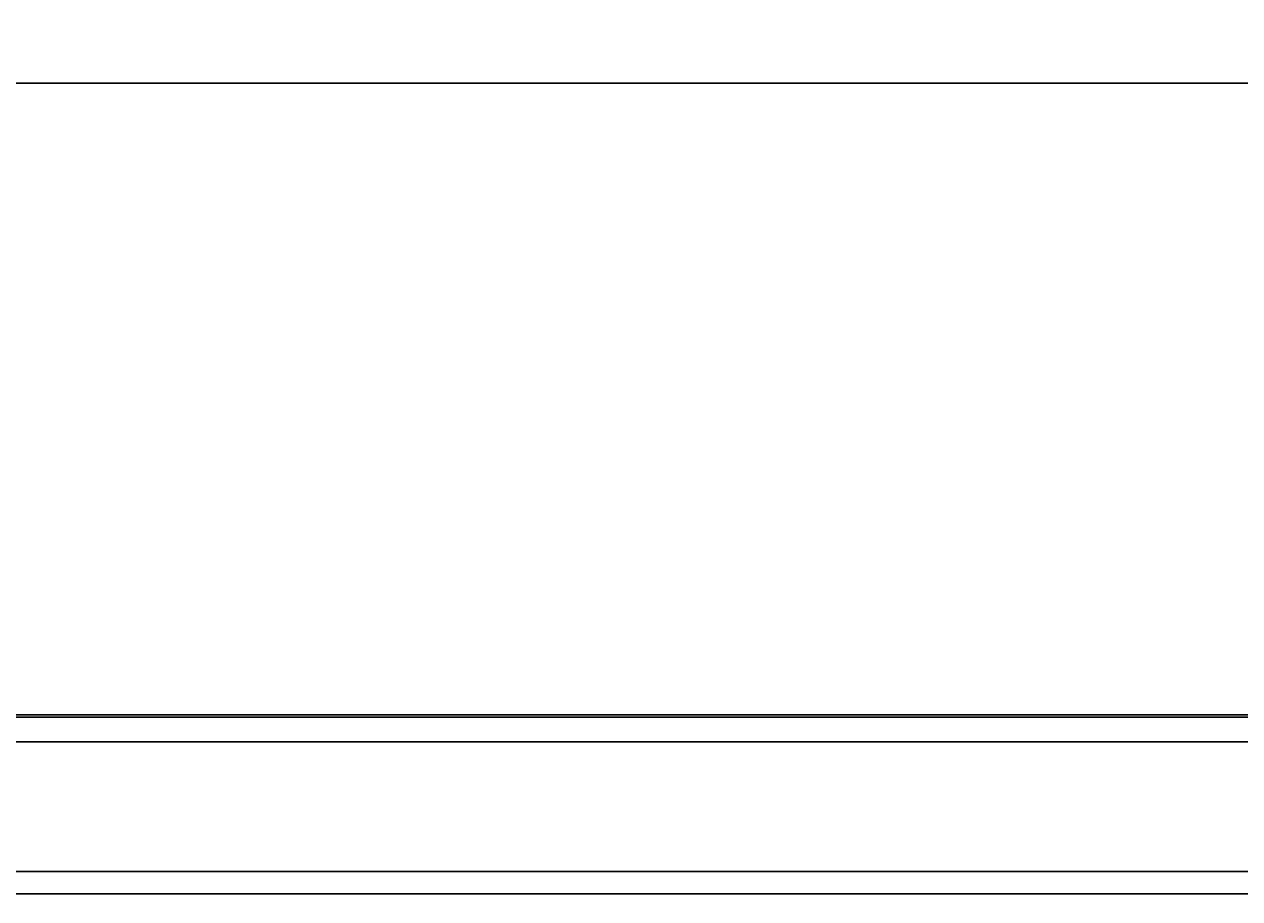
# Model space of a CAD drawing. Units: inches. Extents: x 35362 to 73946, y 43607 to 67532.
# Tile 11 of 134: x 40793 to 43509, y 48909 to 50863. Entities that reach past the tile are written whole.
import ezdxf

# ---------------------------------------------------------------- set-up
doc = ezdxf.new("R2010")
doc.units = ezdxf.units.IN
doc.header["$MEASUREMENT"] = 0
doc.layers.add('A-ANNO-DIMS', color=2, linetype='Continuous', lineweight=18)
doc.layers.add('E-WIRE', color=3, linetype='Continuous', lineweight=25)
doc.styles.get("Standard").update_dxf_attribs({"font": 'arial.ttf'})
doc.dimstyles.get("Standard").update_dxf_attribs({"dimtxt": 0.18, "dimasz": 0.18, "dimexe": 0.18, "dimexo": 0.0625, "dimgap": 0.09, "dimtad": 0, "dimtih": 1, "dimtoh": 1, "dimdec": 4, "dimzin": 0, "dimdsep": 46, "dimtxsty": 'Standard', "dimcen": 0.09, "dimadec": 0, "dimazin": 0, "dimtfac": 1, "dimtdec": 4, "dimtofl": 0, "dimtmove": 0, "dimatfit": 3, "dimfxl": 1, "dimtolj": 1, "dimtzin": 0, "dimarcsym": 0})

# ---------------------------------------------------------------- blocks, each defined once
blk = doc.blocks.new('*D40')
at = {"layer": 'A-ANNO-DIMS', "color": 0, "lineweight": -2, "transparency": 16777216}
for p, q in [((56873.5, 53351.5), (35361.8, 53351.5)), ((35361.9, 53351.3), (35361.9, 51333.3)), ((35361.9, 49314.8), (35361.9, 51332.9)), ((51806.5, 49314.7), (35361.8, 49314.7))]:
    blk.add_line(p, q, dxfattribs=at)
at = {"layer": 'A-ANNO-DIMS', "color": 0, "transparency": 16777216}
for points in [[(35361.9, 53351.3), (35362, 53351.3), (35361.9, 53351.5)], [(35361.9, 49314.8), (35362, 49314.8), (35361.9, 49314.7)]]:
    blk.add_solid(points, dxfattribs=at)
at = {"layer": 'Defpoints', "color": 0, "transparency": 16777216}
for p in [(35361.9, 53351.5), (56873.6, 53351.5), (51806.5, 49314.7)]:
    blk.add_point(p, dxfattribs=at)
at = {"layer": 'A-ANNO-DIMS', "color": 0, "transparency": 16777216, "insert": (35361.9, 51333.1), "char_height": 0.18, "attachment_point": 5}
blk.add_mtext('\\A1;4036.9', dxfattribs=at)
blk = doc.blocks.new('*D67')
at = {"layer": 'A-ANNO-DIMS', "color": 0, "lineweight": -2, "transparency": 16777216}
for p, q in [((56873.5, 53351.5), (35361.8, 53351.5)), ((35361.9, 53351.3), (35361.9, 49400.9)), ((35361.9, 45450.1), (35361.9, 49400.5)), ((53793.6, 45449.9), (35361.8, 45449.9))]:
    blk.add_line(p, q, dxfattribs=at)
at = {"layer": 'A-ANNO-DIMS', "color": 0, "transparency": 16777216}
for points in [[(35361.9, 53351.3), (35362, 53351.3), (35361.9, 53351.5)], [(35361.9, 45450.1), (35362, 45450.1), (35361.9, 45449.9)]]:
    blk.add_solid(points, dxfattribs=at)
at = {"layer": 'Defpoints', "color": 0, "transparency": 16777216}
for p in [(35361.9, 53351.5), (56873.6, 53351.5), (53793.6, 45449.9)]:
    blk.add_point(p, dxfattribs=at)
at = {"layer": 'A-ANNO-DIMS', "color": 0, "transparency": 16777216, "insert": (35361.9, 49400.7), "char_height": 0.18, "attachment_point": 5}
blk.add_mtext('\\A1;7901.6', dxfattribs=at)
blk = doc.blocks.new('*D84')
at = {"layer": 'A-ANNO-DIMS', "color": 0, "lineweight": -2, "transparency": 16777216}
for p, q in [((55540.2, 49259.9), (35361.8, 49259.9)), ((35361.9, 49259.8), (35361.9, 49115.1)), ((35361.9, 48970.2), (35361.9, 49114.8)), ((55540.2, 48970), (35361.8, 48970))]:
    blk.add_line(p, q, dxfattribs=at)
at = {"layer": 'A-ANNO-DIMS', "color": 0, "transparency": 16777216}
for points in [[(35361.9, 49259.8), (35362, 49259.8), (35361.9, 49259.9)], [(35361.9, 48970.2), (35362, 48970.2), (35361.9, 48970)]]:
    blk.add_solid(points, dxfattribs=at)
at = {"layer": 'Defpoints', "color": 0, "transparency": 16777216}
for p in [(35361.9, 49259.9), (55540.3, 49259.9), (55540.3, 48970)]:
    blk.add_point(p, dxfattribs=at)
at = {"layer": 'A-ANNO-DIMS', "color": 0, "transparency": 16777216, "insert": (35361.9, 49115), "char_height": 0.18, "attachment_point": 5}
blk.add_mtext('\\A1;289.96', dxfattribs=at)
blk = doc.blocks.new('*D86')
at = {"layer": 'A-ANNO-DIMS', "color": 0, "lineweight": -2, "transparency": 16777216}
for p, q in [((51285.5, 49320.1), (35361.8, 49320.1)), ((35361.9, 49319.9), (35361.9, 49120.3)), ((35361.9, 48920.3), (35361.9, 49119.9)), ((51285.5, 48920.1), (35361.8, 48920.1))]:
    blk.add_line(p, q, dxfattribs=at)
at = {"layer": 'A-ANNO-DIMS', "color": 0, "transparency": 16777216}
for points in [[(35361.9, 49319.9), (35362, 49319.9), (35361.9, 49320.1)], [(35361.9, 48920.3), (35362, 48920.3), (35361.9, 48920.1)]]:
    blk.add_solid(points, dxfattribs=at)
at = {"layer": 'Defpoints', "color": 0, "transparency": 16777216}
for p in [(35361.9, 49320.1), (51285.6, 49320.1), (51285.6, 48920.1)]:
    blk.add_point(p, dxfattribs=at)
at = {"layer": 'A-ANNO-DIMS', "color": 0, "transparency": 16777216, "insert": (35361.9, 49120.1), "char_height": 0.18, "attachment_point": 5}
blk.add_mtext('\\A1;400.0', dxfattribs=at)

msp = doc.modelspace()

# ---------------------------------------------------------------- linework, layer by layer
at = {"layer": 'E-WIRE'}
msp.add_line((38575.774, 50731.821), (54718.752, 50731.821), dxfattribs=at)

# ---------------------------------------------------------------- dimensions: what is measured, and where the dimension line sits
at = {"layer": 'A-ANNO-DIMS'}
for base, p1, p2, override, picture, middle in [((35361.949, 53351.529), (51806.517, 49314.669), (56873.602, 53351.529), {"dimdec": 1, "dimlfac": 1, "dimrnd": 0, "dimzin": 0, "dimdsep": 46, "dimlunit": 2}, '*D40', (35361.949, 51333.099)), ((35361.949, 53351.529), (53793.638, 45449.894), (56873.602, 53351.529), {"dimdec": 1, "dimlfac": 1, "dimrnd": 0, "dimzin": 0, "dimdsep": 46, "dimlunit": 2}, '*D67', (35361.949, 49400.712)), ((35361.949, 49320.079), (51285.595, 48920.079), (51285.595, 49320.079), {"dimdec": 1, "dimlfac": 1, "dimrnd": 0, "dimzin": 0, "dimdsep": 46, "dimlunit": 2}, '*D86', (35361.949, 49120.079)), ((35361.9491, 49259.9353), (55540.2972, 48969.9796), (55540.2972, 49259.9353), {"dimdec": 2, "dimlfac": 1, "dimrnd": 0, "dimzin": 0, "dimdsep": 46, "dimlunit": 2}, '*D84', (35361.9491, 49114.9575))]:
    dim = msp.add_linear_dim(base=base, p1=p1, p2=p2, angle=90, dimstyle='Standard', override=override, dxfattribs=at)
    dim.commit()
    dim.dimension.update_dxf_attribs({"geometry": picture, "text_midpoint": middle})

doc.saveas('drawing.dxf')
